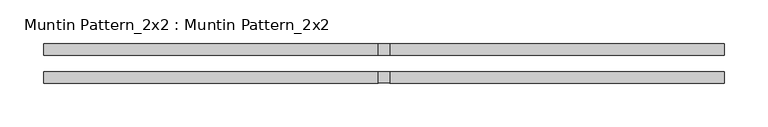
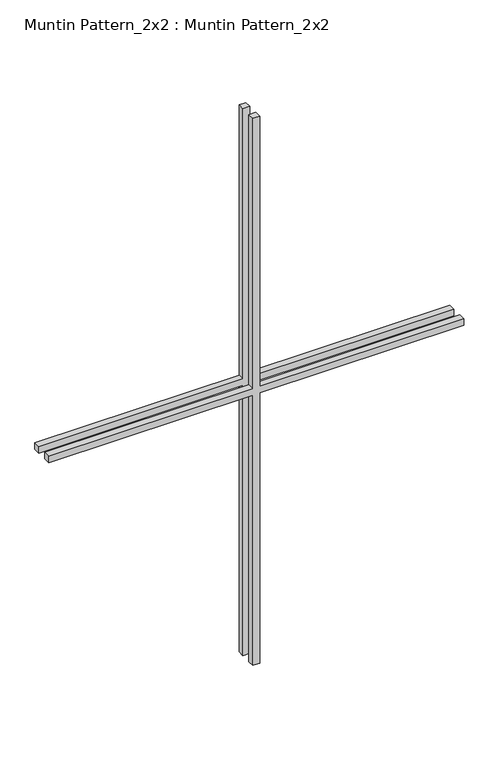
"""IFC4 building model written with IfcOpenShell, lengths in millimetres: proxy geometry, Muntin Pattern_2x2 : Muntin Pattern_2x2."""

from ifc_helpers import new_model, si_unit, frame, origin, place, context, project, spatial, polyline, outline, extrude, source, transform, mapped, element, save


def muntin_pattern_2x2_muntin_pattern_2x2_95b57395(model_context):
    return source(origin(), model_context, "Body", "SweptSolid", [
        extrude(outline(polyline([(546.1, -6.35), (546.1, -387.35), (533.4, -387.35), (533.4, -6.35), (0.0, -6.35), (0.0, 6.35), (533.4, 6.35), (533.4, 387.35), (546.1, 387.35), (546.1, 6.35), (1079.5, 6.35), (1079.5, -6.35), (546.1, -6.35)])), frame((0.0, 9.525, 0.0), z_axis=(0.0, 1.0, 0.0), x_axis=(0.0, 0.0, 1.0)), (0.0, 0.0, 1.0), 12.7),
        extrude(outline(polyline([(546.1, -6.35), (546.1, -387.35), (533.4, -387.35), (533.4, -6.35), (0.0, -6.35), (0.0, 6.35), (533.4, 6.35), (533.4, 387.35), (546.1, 387.35), (546.1, 6.35), (1079.5, 6.35), (1079.5, -6.35), (546.1, -6.35)])), frame((0.0, -22.225, 0.0), z_axis=(0.0, 1.0, 0.0), x_axis=(0.0, 0.0, 1.0)), (0.0, 0.0, 1.0), 12.7),
    ])


if __name__ == "__main__":
    model = new_model("IFC4")
    model_context = context("Model", 3, world=origin())
    ifc_project = project(units=[si_unit("LENGTHUNIT", "METRE", prefix="MILLI")], contexts=[model_context])
    site = spatial("IfcSite", under=ifc_project)
    building = spatial("IfcBuilding", under=site)
    placement = place(None, origin())
    muntin_pattern_2x2_muntin_pattern_2x2_shape = muntin_pattern_2x2_muntin_pattern_2x2_95b57395(model_context)
    element("IfcBuildingElementProxy", 1, Name="Muntin Pattern_2x2 : Muntin Pattern_2x2", ObjectType="Muntin Pattern_2x2 : Muntin Pattern_2x2", at=placement, inside=building, context=model_context, shape_type="MappedRepresentation", body=[
        mapped(muntin_pattern_2x2_muntin_pattern_2x2_shape, transform((0.0, 0.0, 0.0), x_axis=(1.0, 0.0, 0.0), y_axis=(0.0, 1.0, 0.0), z_axis=(0.0, 0.0, 1.0))),
    ])
    save(model, "model.ifc")

# Revit data of these elements
# Type "Muntin Pattern_2x2 : Muntin Pattern_2x2"
#   Width [instance default] = 4' - 0"
#   Thickness = 0' - 0 1/2"
#   Height [instance default] = 4' - 0"
#   Distance = 0' - 0 3/4"
#   Interior Material [instance default] = none
#   Exterior Material [instance default] = none
#   Default Elevation = 0
# Element 1 (IfcBuildingElementProxy, "Muntin Pattern_2x2 : Muntin Pattern_2x2")
#   Width = 2' - 6 1/2"
#   Height = 3' - 6 1/2"
#   Interior Material = Wood - Stained
#   Exterior Material = Clad - White
#   Materials on its faces: "Clad - White", "Wood - Stained"
# Materials
#   "Clad - White": class "Wood", colour RGB 242 242 238, transparency 0, Cost = 0
#   "Wood - Stained": class "Wood", colour RGB 224 178 126, transparency 0, Cost = 0
